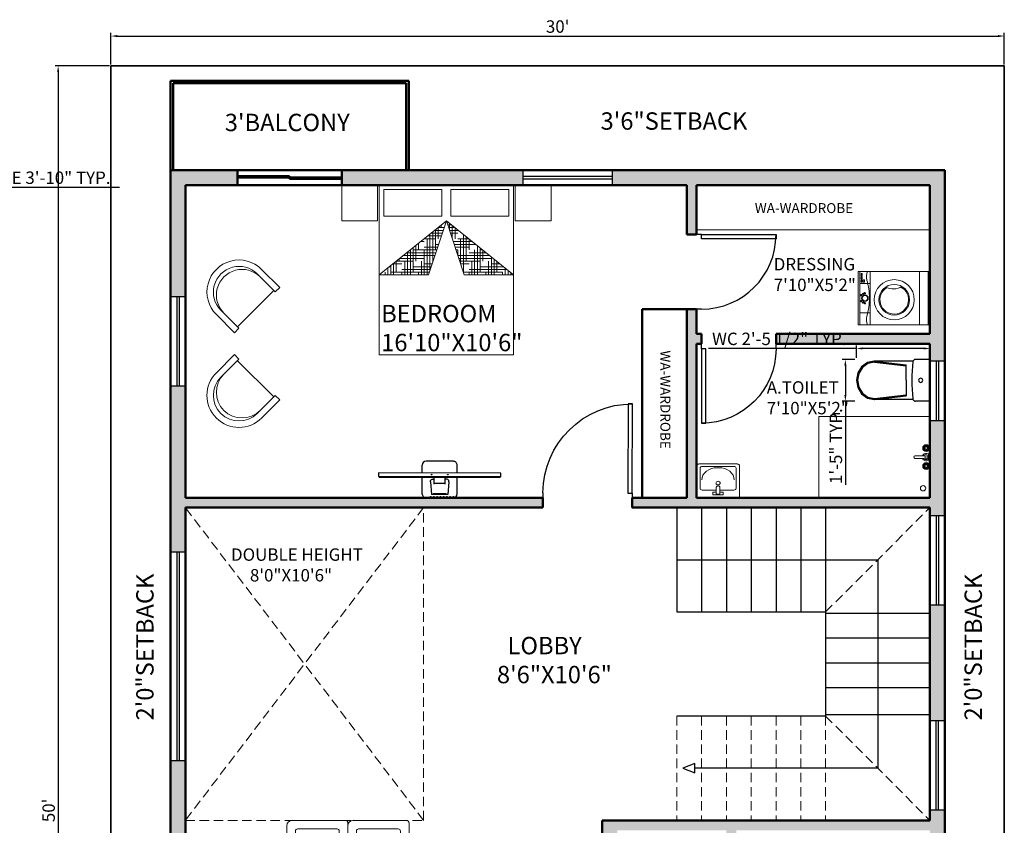
# Model space of a CAD drawing. Units: inches. Extents: x 2638 to 4577, y 1946 to 2619.
# Tile 6 of 8: x 3050 to 3447, y 2294 to 2619. Entities that reach past the tile are written whole.
import ezdxf

# ---------------------------------------------------------------- set-up
doc = ezdxf.new("R2010")
doc.units = ezdxf.units.IN
doc.linetypes.add('DASHED', pattern=[19.05, 12.7, -6.35])
for name, color, linetype, lineweight in [('A-ANNO-DIMS', 2, 'Continuous', 18), ('A-ANNO-TEXT', 7, 'Continuous', 25), ('A-AREA-IDEN', 7, 'Continuous', 25), ('A-DOOR', 4, 'Continuous', 25), ('A-FLOR-FIXT', 8, 'Continuous', 18), ('A-FLOR-OVHD', 8, 'DASHED', 18), ('A-FLOR-STRS', 3, 'Continuous', 25), ('A-FURN', 8, 'Continuous', 18), ('A-GLAZ', 4, 'Continuous', 25), ('A-WALL', 7, 'Continuous', 50), ('A-WALL-PATT', 8, 'Continuous', 13), ('C-PROP', 1, 'Continuous', 35)]:
    doc.layers.add(name, color=color, linetype=linetype, lineweight=lineweight)
doc.layers.add('SANTEH', color=7, linetype='Continuous')
doc.layers.add('window', color=130, linetype='Continuous')
doc.styles.get("Standard").update_dxf_attribs({"font": 'arial.ttf'})
doc.dimstyles.new('ISO-25', dxfattribs={"dimtxt": 5, "dimasz": 2.5, "dimexe": 1.25, "dimexo": 0.625, "dimtad": 1, "dimdec": 1, "dimlunit": 3, "dimtxsty": 'Standard', "dimcen": 2.5, "dimclrt": 1, "dimadec": 0, "dimazin": 0, "dimtfac": 1, "dimtdec": 1, "dimtmove": 0, "dimatfit": 3, "dimfxl": 1, "dimarcsym": 0})

# ---------------------------------------------------------------- blocks, each defined once
blk = doc.blocks.new('*D6')
at = {"layer": 'A-ANNO-DIMS', "color": 0, "lineweight": -2, "transparency": 16777216}
for p, q in [((3086.99, 2600.78), (3086.99, 2613.44)), ((3089.49, 2612.19), (3444.49, 2612.19)), ((3446.99, 2600.78), (3446.99, 2613.44))]:
    blk.add_line(p, q, dxfattribs=at)
at = {"layer": 'A-ANNO-DIMS', "color": 0, "transparency": 16777216}
for points in [[(3089.49, 2612.61), (3089.49, 2611.77), (3086.99, 2612.19)], [(3444.49, 2612.61), (3444.49, 2611.77), (3446.99, 2612.19)]]:
    blk.add_solid(points, dxfattribs=at)
at = {"layer": 'Defpoints', "color": 0, "transparency": 16777216}
for p in [(3446.99, 2612.19), (3086.99, 2600.16), (3446.99, 2600.16)]:
    blk.add_point(p, dxfattribs=at)
at = {"layer": 'A-ANNO-DIMS', "color": 0, "transparency": 16777216, "insert": (3266.99, 2615.37), "char_height": 5, "attachment_point": 5}
blk.add_mtext("30'", dxfattribs=at)
blk = doc.blocks.new('*D7')
at = {"layer": 'A-ANNO-DIMS', "color": 0, "lineweight": -2, "transparency": 16777216}
for p, q in [((3086.37, 2600.16), (3064.44, 2600.16)), ((3065.69, 2597.66), (3065.69, 2002.66)), ((3086.37, 2000.16), (3064.44, 2000.16))]:
    blk.add_line(p, q, dxfattribs=at)
at = {"layer": 'A-ANNO-DIMS', "color": 0, "transparency": 16777216}
for points in [[(3065.28, 2597.66), (3066.11, 2597.66), (3065.69, 2600.16)], [(3065.28, 2002.66), (3066.11, 2002.66), (3065.69, 2000.16)]]:
    blk.add_solid(points, dxfattribs=at)
at = {"layer": 'Defpoints', "color": 0, "transparency": 16777216}
for p in [(3086.99, 2600.16), (3065.69, 2000.16), (3086.99, 2000.16)]:
    blk.add_point(p, dxfattribs=at)
at = {"layer": 'A-ANNO-DIMS', "color": 0, "transparency": 16777216, "insert": (3062.52, 2300.16), "char_height": 5, "attachment_point": 5, "rotation": 90}
blk.add_mtext("50'", dxfattribs=at)
blk = doc.blocks.new('*U5')
for p, q in [((0, 0), (0, -6)), ((30, 0), (30, -6))]:
    blk.add_line(p, q)
blk.add_lwpolyline([(0, 0), (0, 30), (1.75, 30), (1.75, 0)], close=True)
blk.add_arc((0, 0), 30, 0, 90)
blk = doc.blocks.new('*U4')
for p, q in [((0, 0), (0, -6)), ((36, 0), (36, -6))]:
    blk.add_line(p, q)
blk.add_lwpolyline([(0, 0), (0, 36), (1.75, 36), (1.75, 0)], close=True)
blk.add_arc((0, 0), 36, 0, 90)
blk = doc.blocks.new('Rac7')
at = {"color": 0}
for p, q in [((-39501, -24232), (-39501, -23830)), ((-39474, -23808), (-38988, -23808)), ((-39457, -23859), (-39457, -24115)), ((-39032, -23838), (-39430, -23838)), ((-39221, -23855), (-39241, -23855)), ((-39005, -24115), (-39005, -23859)), ((-39005, -23859), (-39005, -23859)), ((-38961, -23830), (-38961, -24232)), ((-39253, -24186), (-39253, -24094)), ((-39209, -24186), (-39209, -24094)), ((-38961, -24232), (-39501, -24232)), ((-39430, -24136), (-39253, -24136)), ((-39297, -24164), (-39253, -24164)), ((-39297, -24194), (-39297, -24164)), ((-39165, -24194), (-39297, -24194)), ((-39253, -24186), (-39209, -24186)), ((-39209, -24136), (-39032, -24136)), ((-39209, -24164), (-39165, -24164)), ((-39165, -24164), (-39165, -24194))]:
    blk.add_line(p, q, dxfattribs=at)
at = {"color": 0, "extrusion": (0, 0, -1)}
for centre, major_axis, start_param, end_param in [((-39474, -23830), (-27, 0), 0, 1.570796), ((-39430, -23859), (-27, 0), 0, 1.570796), ((-39241, -24007), (-194, 0), 0, 1.570796), ((-39221, -24007), (-194, 0), 1.570796, 3.141593), ((-39032, -23859), (-27, 0), 1.570796, 3.141593), ((-38988, -23830), (-27, 0), 1.570796, 3.141593), ((-39430, -24115), (-27, 0), -1.570796, 0), ((-39231, -24104), (-25.3, 0), 0.552816, 2.588777), ((-39032, -24115), (-27, 0), -3.141593, -1.570796)]:
    blk.add_ellipse(centre, major_axis=major_axis, ratio=0.785714, start_param=start_param, end_param=end_param, dxfattribs=at)
blk.add_ellipse((-39231, -24048), major_axis=(-27.9, 0), ratio=0.785714, dxfattribs=at)
blk = doc.blocks.new('WC 2 Symb_109')
at = {"layer": 'SANTEH'}
for p, q in [((0, 0), (0, 380)), ((0, 380), (132.4, 380)), ((153.6, 364.9), (506.8, 364.9)), ((506.3, 364.9), (215.7, 330.9)), ((506.3, 356), (215.7, 322)), ((215.7, 190), (215.7, 330.9)), ((215.7, 190), (215.7, 49.1)), ((153.8, 15.1), (506.8, 15.1)), ((506.3, 24), (215.7, 58)), ((506.3, 15.1), (215.7, 49.1)), ((0, 0), (132.4, 0))]:
    blk.add_line(p, q, dxfattribs=at)
for points in [[(154.6, 360.1), (153.9, 364.1), (152.3, 367.9), (150.2, 371.3), (147.4, 374.3), (144.1, 376.7), (140.5, 378.5), (136.5, 379.6), (132.4, 380)], [(154.6, 19.7), (158.6, 62.1), (161.4, 104.7), (163.1, 147.3), (163.7, 189.9), (163.1, 232.5), (161.4, 275.1), (158.6, 317.7), (154.6, 360.1)], [(506.8, 15.1), (569.2, 28.4), (622.2, 66.3), (657.6, 123.1), (670, 190), (657.6, 256.9), (622.2, 313.7), (569.2, 351.6), (506.8, 364.9)], [(506.3, 24), (565.5, 36.6), (615.7, 72.6), (649.2, 126.5), (661, 190), (649.2, 253.5), (615.7, 307.4), (565.5, 343.4), (506.3, 356)], [(132.4, 0), (136.5, 0.4), (140.4, 1.5), (144.1, 3.2), (147.3, 5.6), (150.1, 8.6), (152.3, 12), (153.8, 15.7), (154.6, 19.7)]]:
    blk.add_lwpolyline(points, dxfattribs=at)
blk.add_lwpolyline([(83.6, 208.5), (70.4, 203.1), (64.9, 190), (70.4, 176.9), (83.6, 171.5), (96.8, 176.9), (102.2, 190), (96.8, 203.1)], close=True, dxfattribs=at)
blk = doc.blocks.new('Faucet - Bathroom top')
for p, q in [((-4.107, 0.125), (-4.375, 0.125)), ((-3.75, 0.4788), (-3.75, 0.75)), ((-3.5, 0.482), (-3.5, 0.75)), ((-3.1461, 0.125), (-2.875, 0.125)), ((3.143, 0.125), (2.875, 0.125)), ((3.5, 0.4788), (3.5, 0.75)), ((3.75, 0.482), (3.75, 0.75)), ((4.1039, 0.125), (4.375, 0.125)), ((-4.1039, -0.125), (-4.375, -0.125)), ((-3.75, -0.4821), (-3.75, -0.75)), ((-3.5, -0.4789), (-3.5, -0.75)), ((-3.143, -0.125), (-2.875, -0.125)), ((-0.5, -0.8639), (-0.5, -4.5)), ((0.5, -4.5), (0.5, -0.8631)), ((3.1461, -0.125), (2.875, -0.125)), ((3.5, -0.4821), (3.5, -0.75)), ((3.75, -0.4789), (3.75, -0.75)), ((4.107, -0.125), (4.375, -0.125))]:
    blk.add_line(p, q)
for centre, radius in [((-3.625, 0), 1.375), ((-4.625, 0), 0.2795), ((-3.625, 0), 0.5), ((-3.625, 1), 0.2795), ((-2.625, 0), 0.2795), ((0, 0), 0.5), ((3.625, 0), 1.375), ((2.625, 0), 0.2795), ((3.625, 0), 0.5), ((3.625, 1), 0.2795), ((4.625, 0), 0.2795), ((-3.625, -1), 0.2795), ((3.625, -1), 0.2795)]:
    blk.add_circle(centre, radius)
for centre, radius, start, end in [((-3.625, 0), 1, 105.2407, 164.2093), ((-3.625, 0), 1, 16.44125, 74.07887), ((0, 0), 1.5, 289.6514, 250.3603), ((0, 0), 1, 300.3431, 239.7554), ((3.625, 0), 1, 106.12, 164.0884), ((3.625, 0), 1, 16.23422, 73.90469), ((-3.625, 0), 1, 196.2342, 253.9047), ((-3.625, 0), 1, 286.12, 344.0884), ((3.625, 0), 1, 196.4413, 254.0789), ((3.625, 0), 1, 285.2407, 344.2093), ((0, -4.5), 0.5, 180, 0)]:
    blk.add_arc(centre, radius, start, end)
blk = doc.blocks.new('*X22')
at = {"color": 0}
for p, q in [((20.188, 14.75), (20.188, 14.767)), ((20.199, 14.781), (20.277, 14.781)), ((20.25, 14.812), (20.277, 14.812)), ((20.094, 14.375), (20.094, 14.65)), ((20.098, 14.656), (20.125, 14.656)), ((20.124, 14.688), (20.25, 14.688)), ((20.125, 14.5), (20.125, 14.689)), ((20.149, 14.719), (20.277, 14.719)), ((20.156, 14.625), (20.156, 14.728)), ((20.174, 14.75), (20.277, 14.75)), ((20.25, 14.319), (20.25, 14.75)), ((20.023, 14.562), (20.277, 14.562)), ((20.031, 14.247), (20.031, 14.573)), ((20.062, 14.257), (20.062, 14.612)), ((20.125, 14.594), (20.277, 14.594)), ((20.219, 14.309), (20.219, 14.625)), ((20.25, 14.625), (20.277, 14.625)), ((19.922, 14.438), (20, 14.438)), ((19.948, 14.469), (20.125, 14.469)), ((19.973, 14.5), (20.25, 14.5)), ((19.998, 14.531), (20.277, 14.531)), ((20, 14.237), (20, 14.5)), ((20.188, 14.299), (20.188, 14.5)), ((20.25, 14.438), (20.277, 14.438)), ((19.844, 14.185), (19.844, 14.34)), ((19.875, 14.25), (19.875, 14.379)), ((19.875, 14.344), (20.277, 14.344)), ((19.906, 14.375), (19.906, 14.417)), ((19.969, 14.226), (19.969, 14.375)), ((20, 14.375), (20.277, 14.375)), ((20.125, 14.406), (20.277, 14.406)), ((20.156, 14.288), (20.156, 14.375)), ((19.746, 14.219), (19.875, 14.219)), ((19.75, 14.154), (19.75, 14.223)), ((19.772, 14.25), (20, 14.25)), ((19.781, 14.164), (19.781, 14.262)), ((19.797, 14.281), (20.125, 14.281)), ((19.812, 14.174), (19.812, 14.301)), ((19.822, 14.312), (20.229, 14.312)), ((19.938, 14.216), (19.938, 14.25)), ((19.719, 14.073), (19.719, 14.114)), ((19.721, 14.188), (19.75, 14.188)), ((19.75, 14.034), (19.75, 14.103)), ((19.702, 14.094), (19.779, 14.094)), ((19.727, 14.062), (19.873, 14.062)), ((19.752, 14.031), (19.875, 14.031)), ((19.781, 13.995), (19.781, 14.093)), ((19.812, 14), (19.812, 14.082)), ((19.875, 13.878), (19.875, 14)), ((19.906, 13.84), (19.906, 14.051)), ((19.938, 13.801), (19.938, 14.041)), ((19.969, 13.875), (19.969, 14.031)), ((20, 14), (20, 14.02)), ((20, 14), (20.061, 14)), ((20.062, 13.645), (20.062, 14)), ((20.094, 13.625), (20.094, 13.989)), ((19.827, 13.938), (20.25, 13.938)), ((19.853, 13.906), (20.125, 13.906)), ((19.875, 13.969), (20.156, 13.969)), ((19.878, 13.875), (20, 13.875)), ((20.031, 13.684), (20.031, 13.875)), ((20.125, 13.75), (20.125, 13.979)), ((20.156, 13.875), (20.156, 13.969)), ((20.219, 13.451), (20.219, 13.875)), ((20.25, 13.5), (20.25, 13.937)), ((20.25, 13.875), (20.277, 13.875)), ((19.953, 13.781), (20.277, 13.781)), ((20, 13.812), (20.277, 13.812)), ((20.125, 13.844), (20.277, 13.844)), ((19.978, 13.75), (20.25, 13.75)), ((20, 13.723), (20, 13.75)), ((20.003, 13.719), (20.125, 13.719)), ((20.125, 13.656), (20.277, 13.656)), ((20.188, 13.49), (20.188, 13.75)), ((20.25, 13.688), (20.277, 13.688)), ((20.079, 13.625), (20.277, 13.625)), ((20.104, 13.594), (20.277, 13.594)), ((20.129, 13.562), (20.25, 13.562)), ((20.156, 13.529), (20.156, 13.625)), ((20.205, 13.469), (20.277, 13.469)), ((20.23, 13.438), (20.277, 13.438)), ((20.25, 13.5), (20.277, 13.5)), ((20.255, 13.406), (20.277, 13.406))]:
    blk.add_line(p, q, dxfattribs=at)
blk = doc.blocks.new('MAT-P02')
for p, q in [((-1.17, 0), (-1.17, -0.4)), ((-1.17, 0), (-0.77, 0)), ((-0.77, 0), (-0.77, -0.4)), ((-0.75, 0), (0.75, 0)), ((-0.75, 0), (-0.75, -1.9)), ((0.75, 0), (0.75, -1.9)), ((0.77, 0), (1.17, 0)), ((0.77, 0), (0.77, -0.4)), ((1.17, 0), (1.17, -0.4)), ((-0.7, -0.05), (-0.7, -0.35)), ((-0.7, -0.05), (-0.05, -0.05)), ((-0.05, -0.35), (-0.05, -0.05)), ((0.05, -0.05), (0.7, -0.05)), ((0.05, -0.35), (0.05, -0.05)), ((0.7, -0.05), (0.7, -0.35)), ((-1.17, -0.4), (-0.77, -0.4)), ((-0.75, -1.003), (0, -0.4)), ((0, -0.4), (-0.75, -1.003)), ((-0.7, -0.35), (-0.05, -0.35)), ((0, -0.4), (-0.2, -1.003)), ((0, -0.4), (0.2, -1.003)), ((0, -0.4), (0.75, -1.003)), ((0.05, -0.35), (0.7, -0.35)), ((0.77, -0.4), (1.17, -0.4)), ((-0.75, -1.003), (-0.2, -1.003)), ((0.2, -1.003), (0.75, -1.003)), ((0.75, -1.9), (-0.75, -1.9))]:
    blk.add_line(p, q)
at = {"xscale": -1, "rotation": 90}
blk.add_blockref('*X22', (14.128, 19.274), dxfattribs=at)
blk = doc.blocks.new('12PSTG07')
at = {"color": 0, "linetype": 'ByBlock'}
for p, q in [((0, 15), (-12, 15)), ((0, 12), (0, 15)), ((-12, 12), (0, 12)), ((-1, -12), (-1, 12)), ((-12, -12), (0, -12)), ((0, -12), (0, -15)), ((0, -15), (-12, -15))]:
    blk.add_line(p, q, dxfattribs=at)
for centre, radius in [((-12, 0), 15), ((-12, 0), 12), ((-10, 0), 12)]:
    blk.add_arc(centre, radius, 90, 270, dxfattribs=at)
blk = doc.blocks.new('sofa-27')
at = {"color": 0, "linetype": 'ByBlock'}
for p, q in [((-0.059, 0.059), (-0.059, 0.49)), ((0.035, 0.118), (0.035, 0.461)), ((0.094, 0.52), (0.459, 0.52)), ((0.518, 0.118), (0.518, 0.461)), ((0.613, 0.03), (0.613, 0.49)), ((0.583, 0), (0, 0)), ((0.494, 0.094), (0.059, 0.094))]:
    blk.add_line(p, q, dxfattribs=at)
for centre, radius, start, end in [((-0.03, 0.49), 0.0295, 90, 180), ((-0.024, 0.461), 0.0591, 360, 90), ((0.094, 0.461), 0.0591, 90, 180), ((0.459, 0.461), 0.0591, 0, 90), ((0.577, 0.461), 0.0591, 90, 180), ((0.583, 0.49), 0.0295, 0, 90), ((0.059, 0.118), 0.0236, 180, 270), ((0.494, 0.118), 0.0236, 270, 0), ((0, 0.059), 0.0591, 180, 270), ((0.583, 0.03), 0.0295, 270, 0)]:
    blk.add_arc(centre, radius, start, end, dxfattribs=at)
blk = doc.blocks.new('TV')
at = {"color": 0}
for p, q in [((3967.27, 1784.85), (3967.05, 1784.65)), ((3967.76, 1763.68), (3967.54, 1763.86))]:
    blk.add_line(p, q, dxfattribs=at)
at = {"layer": 'window'}
for p, q in [((3967.54, 1763.86), (3967.05, 1784.65)), ((3964.41, 1777.23), (3967.22, 1777.3)), ((3968.01, 1777.32), (3969.36, 1777.35)), ((3966.53, 1775.82), (3964.33, 1775.61)), ((3964.34, 1775.34), (3964.45, 1775.34)), ((3964.34, 1775.31), (3964.43, 1775.32)), ((3966.14, 1775.2), (3967.01, 1775.22)), ((3966.14, 1775.18), (3967.27, 1775.2)), ((3966.14, 1775.18), (3966.14, 1775.2)), ((3966.3, 1773.29), (3966.26, 1775.18)), ((3966.19, 1773.28), (3967.31, 1773.31)), ((3966.19, 1773.26), (3967.05, 1773.28)), ((3966.19, 1773.26), (3966.19, 1773.28)), ((3964.39, 1773.06), (3964.48, 1773.06)), ((3964.39, 1773.04), (3964.5, 1773.04)), ((3966.61, 1772.66), (3964.4, 1772.77)), ((3964.55, 1771.15), (3967.36, 1771.22)), ((3968.15, 1771.24), (3969.5, 1771.27))]:
    blk.add_line(p, q, dxfattribs=at)
for points in [[(3968.33, 1763.69), (3967.83, 1784.86), (3967.27, 1784.85), (3967.76, 1763.68), (3968.33, 1763.69)], [(3963.86, 1771.81), (3963.75, 1776.54)], [(3970.16, 1771.96), (3970.05, 1776.69)], [(3964.4, 1772.77), (3964.33, 1775.61)], [(3964.48, 1773.06), (3964.43, 1775.32)], [(3964.5, 1773.04), (3964.45, 1775.34)]]:
    blk.add_lwpolyline(points, dxfattribs=at)
for points in [[(3966.53, 1775.82, -0.263666), (3966.93, 1775.69), (3967, 1775.57), (3967.01, 1775.22)], [(3966.61, 1772.66, 0.263666), (3967, 1772.81), (3967.06, 1772.93), (3967.05, 1773.28)]]:
    blk.add_lwpolyline(points, format="xyb", dxfattribs=at)
for centre, radius in [((3963.91, 1775.73), 0.0679), ((3963.93, 1775.17), 0.0679), ((3967.77, 1775.68), 0.0451), ((3963.94, 1774.6), 0.0679), ((3963.95, 1774.04), 0.0679), ((3963.97, 1773.48), 0.0679), ((3963.98, 1772.92), 0.0679), ((3963.99, 1772.35), 0.0679), ((3964.01, 1771.79), 0.0679), ((3967.83, 1772.86), 0.0451)]:
    blk.add_circle(centre, radius, dxfattribs=at)
for centre, start, end in [((3964.42, 1776.56), 91.3414, 181.3414), ((3969.38, 1776.67), 1.3414, 91.3414), ((3964.53, 1771.83), 181.3414, 271.3414), ((3969.49, 1771.94), 271.3414, 1.3414)]:
    blk.add_arc(centre, 0.676, start, end, dxfattribs=at)
blk = doc.blocks.new('WIN-36')
for p, q in [((2761.41, 2540.16), (2761.41, 2534.16)), ((2797.41, 2540.16), (2797.41, 2534.16)), ((2761.41, 2537.66), (2797.41, 2537.66)), ((2761.41, 2536.66), (2797.41, 2536.66))]:
    blk.add_line(p, q)
blk = doc.blocks.new('WIN-24')
for p, q in [((2905.41, 2558.16), (2905.41, 2552.16)), ((2905.41, 2555.66), (2929.41, 2555.66)), ((2929.41, 2558.16), (2929.41, 2552.16)), ((2905.41, 2554.66), (2929.41, 2554.66))]:
    blk.add_line(p, q)
blk = doc.blocks.new('WIN-84')
for p, q in [((2695.41, 2404.16), (2689.41, 2404.16)), ((2691.91, 2404.16), (2691.91, 2320.16)), ((2692.91, 2404.16), (2692.91, 2320.16)), ((2695.41, 2320.16), (2689.41, 2320.16))]:
    blk.add_line(p, q)
blk = doc.blocks.new('*D69')
at = {"layer": 'A-ANNO-DIMS', "color": 0, "lineweight": -2, "transparency": 16777216}
for p, q in [((3387.38, 2486.31), (3327.72, 2486.31)), ((3387.38, 2482.49), (3387.38, 2487.56)), ((3414.49, 2486.31), (3389.88, 2486.31)), ((3416.99, 2482.49), (3416.99, 2487.56))]:
    blk.add_line(p, q, dxfattribs=at)
at = {"layer": 'A-ANNO-DIMS', "color": 0, "transparency": 16777216}
for points in [[(3389.88, 2486.72), (3389.88, 2485.89), (3387.38, 2486.31)], [(3414.49, 2486.72), (3414.49, 2485.89), (3416.99, 2486.31)]]:
    blk.add_solid(points, dxfattribs=at)
at = {"layer": 'Defpoints', "color": 0, "transparency": 16777216}
for p in [(3387.38, 2486.31), (3387.38, 2481.86), (3416.99, 2481.86)]:
    blk.add_point(p, dxfattribs=at)
at = {"layer": 'A-ANNO-DIMS', "color": 1, "transparency": 16777216, "insert": (3356.3, 2489.52), "char_height": 5, "attachment_point": 5}
blk.add_mtext('WC 2\'-5 1/2" TYP.', dxfattribs=at)
blk = doc.blocks.new('*D70')
at = {"layer": 'A-ANNO-DIMS', "color": 0, "lineweight": -2, "transparency": 16777216}
for p, q in [((3386.76, 2481.86), (3381.69, 2481.86)), ((3382.94, 2479.36), (3382.94, 2467.57)), ((3386.76, 2465.07), (3381.69, 2465.07)), ((3382.94, 2465.07), (3382.94, 2431.32))]:
    blk.add_line(p, q, dxfattribs=at)
at = {"layer": 'A-ANNO-DIMS', "color": 0, "transparency": 16777216}
for points in [[(3382.53, 2479.36), (3383.36, 2479.36), (3382.94, 2481.86)], [(3382.53, 2467.57), (3383.36, 2467.57), (3382.94, 2465.07)]]:
    blk.add_solid(points, dxfattribs=at)
at = {"layer": 'Defpoints', "color": 0, "transparency": 16777216}
for p in [(3387.38, 2481.86), (3382.94, 2465.07), (3387.38, 2465.07)]:
    blk.add_point(p, dxfattribs=at)
at = {"layer": 'A-ANNO-DIMS', "color": 1, "transparency": 16777216, "insert": (3379.76, 2446.94), "char_height": 5, "attachment_point": 5, "rotation": 90}
blk.add_mtext('1\'-5" TYP.', dxfattribs=at)
blk = doc.blocks.new('*D79')
at = {"layer": 'A-ANNO-DIMS', "color": 0, "lineweight": -2, "transparency": 16777216}
for p, q in [((2936.51, 2557.53), (2936.51, 2549.99)), ((2982.61, 2557.53), (2982.61, 2549.99)), ((2939.01, 2551.24), (2980.11, 2551.24)), ((2982.61, 2551.24), (3090.4, 2551.24))]:
    blk.add_line(p, q, dxfattribs=at)
at = {"layer": 'A-ANNO-DIMS', "color": 0, "transparency": 16777216}
for points in [[(2939.01, 2551.66), (2939.01, 2550.82), (2936.51, 2551.24)], [(2980.11, 2551.66), (2980.11, 2550.82), (2982.61, 2551.24)]]:
    blk.add_solid(points, dxfattribs=at)
at = {"layer": 'Defpoints', "color": 0, "transparency": 16777216}
for p in [(2936.51, 2558.16), (2982.61, 2558.16), (2982.61, 2551.24)]:
    blk.add_point(p, dxfattribs=at)
at = {"layer": 'A-ANNO-DIMS', "color": 1, "transparency": 16777216, "insert": (3037.75, 2554.45), "char_height": 5, "attachment_point": 5}
blk.add_mtext('WASHING MACHINE 3\'-10" TYP.', dxfattribs=at)

msp = doc.modelspace()

# ---------------------------------------------------------------- hatches: boundary and pattern name
at = {"layer": 'A-WALL-PATT', "transparency": 33554687}
h = msp.add_hatch(color=256, dxfattribs=at)
h.dxf.hatch_style = 1
h.paths.add_polyline_path([(3116.99, 2552.16), (3137.99, 2552.16), (3137.99, 2558.16), (3110.99, 2558.16), (3110.99, 2507.16), (3116.99, 2507.16)])
h.paths.add_polyline_path([(3252.94, 2558.16), (3179.99, 2558.16), (3179.99, 2552.16), (3194.4, 2552.16), (3252.94, 2552.16)])
h.paths.add_polyline_path([(3422.99, 2558.16), (3288.94, 2558.16), (3288.94, 2552.16), (3318.99, 2552.16), (3318.99, 2532.16), (3322.99, 2532.16), (3322.99, 2552.16), (3416.99, 2552.16), (3416.99, 2492.16), (3354.99, 2492.16), (3354.99, 2488.16), (3416.99, 2488.16), (3416.99, 2481.16), (3422.99, 2481.16)])
h.paths.add_polyline_path([(3422.99, 2457.16), (3416.99, 2457.16), (3416.99, 2426.16), (3372.26, 2426.16), (3322.99, 2426.16), (3322.99, 2439.06), (3322.99, 2488.16), (3324.99, 2488.16), (3324.99, 2492.16), (3322.99, 2492.16), (3322.99, 2502.16), (3318.99, 2502.16), (3318.99, 2426.16), (3297.01, 2426.16), (3296.99, 2422.16), (3416.99, 2422.16), (3416.99, 2418.91), (3422.99, 2418.91)])
h.paths.add_polyline_path([(3146.99, 2104.16), (3116.99, 2104.16), (3116.99, 2116.16), (3110.99, 2116.16), (3110.99, 2098.16), (3146.99, 2098.16)])
h.paths.add_polyline_path([(3236.99, 2104.16), (3224.99, 2104.16), (3224.99, 2098.16), (3236.99, 2098.16)])
h.paths.add_polyline_path([(3290.99, 2252.16), (3284.99, 2252.16), (3284.99, 2104.16), (3278.99, 2104.16), (3278.99, 2098.16), (3284.99, 2098.16), (3284.99, 2000.16), (3290.99, 2000.16), (3290.99, 2018.16), (3314.99, 2018.16), (3314.99, 2024.16), (3290.99, 2024.16)])
h.paths.add_polyline_path([(3422.99, 2060.16), (3416.99, 2060.16), (3416.99, 2024.16), (3392.99, 2024.16), (3392.99, 2018.16), (3422.99, 2018.16)])
h.paths.add_polyline_path([(3422.99, 2244.16), (3416.99, 2244.16), (3416.99, 2220.16), (3372.26, 2220.16), (3338.99, 2220.16), (3338.99, 2222.16), (3334.99, 2222.16), (3334.99, 2216.16), (3416.99, 2216.16), (3416.99, 2096.16), (3422.99, 2096.16)])
h.paths.add_polyline_path([(3422.99, 2300.41), (3416.99, 2300.41), (3416.99, 2296.16), (3284.99, 2296.16), (3284.99, 2288.16), (3290.99, 2288.16), (3290.99, 2292.16), (3334.99, 2292.16), (3334.99, 2252.16), (3338.99, 2252.16), (3338.99, 2292.16), (3416.99, 2292.16), (3416.99, 2268.16), (3422.99, 2268.16)])
h.paths.add_polyline_path([(3422.99, 2382.91), (3416.99, 2382.91), (3416.99, 2336.41), (3422.99, 2336.41)])
h.paths.add_polyline_path([(3260.99, 2426.16), (3116.99, 2426.16), (3116.99, 2471.16), (3110.99, 2471.16), (3110.99, 2404.16), (3116.99, 2404.16), (3116.99, 2422.16), (3260.99, 2422.16)])
h.paths.add_polyline_path([(3116.99, 2320.16), (3110.99, 2320.16), (3110.99, 2152.16), (3116.99, 2152.16)])
h.paths.add_polyline_path([(3192.92, 2481.2), (3252.23, 2481.2), (3252.23, 2507.82), (3192.92, 2507.82)], flags=9)
h.paths.add_polyline_path([(3352.38, 2202.6), (3398.15, 2202.6), (3398.15, 2210.84), (3352.38, 2210.84)], flags=25)
h.paths.add_polyline_path([(3108.13, 2334.43), (3108.13, 2401.53), (3093.19, 2401.53), (3093.19, 2334.43)], flags=9)
h.paths.add_polyline_path([(3441.94, 2334.43), (3441.94, 2401.53), (3426.99, 2401.53), (3426.99, 2334.43)], flags=9)
h.paths.add_polyline_path([(3282.12, 2570.46), (3349.22, 2570.46), (3349.22, 2585.4), (3282.12, 2585.4)], flags=9)
h.paths.add_polyline_path([(3240.15, 2347.41), (3289.11, 2347.41), (3289.11, 2374.03), (3240.15, 2374.03)], flags=9)
h.paths.add_polyline_path([(3169.91, 2226.85), (3224.05, 2226.85), (3224.05, 2253.46), (3169.91, 2253.46)], flags=9)
h.paths.add_polyline_path([(3209.4, 2038.68), (3263.9, 2038.68), (3263.9, 2065.29), (3209.4, 2065.29)], flags=9)
h.paths.add_polyline_path([(3313.05, 2123.44), (3369.27, 2123.44), (3369.27, 2150.05), (3313.05, 2150.05)], flags=9)
h.paths.add_polyline_path([(3359.46, 2259.32), (3395.23, 2259.32), (3395.23, 2278.33), (3359.46, 2278.33)], flags=25)

# ---------------------------------------------------------------- linework, layer by layer
at = {"layer": 'A-FLOR-FIXT'}
for p, q in [((3416.99, 2517.31), (3388.1, 2517.31)), ((3388.1, 2495.85), (3388.1, 2517.31)), ((3388.79, 2495.85), (3388.79, 2517.31)), ((3392.94, 2495.85), (3392.94, 2517.31)), ((3412.84, 2495.85), (3412.84, 2517.31)), ((3416.3, 2495.85), (3416.3, 2517.31)), ((3416.99, 2495.85), (3416.99, 2517.31)), ((3392.94, 2512.46), (3388.79, 2512.46)), ((3392.94, 2500.7), (3388.79, 2500.7)), ((3416.99, 2495.85), (3388.1, 2495.85))]:
    msp.add_line(p, q, dxfattribs=at)
for points in [[(3389.25, 2515.65), (3389.25, 2516.55), (3389.76, 2516.55), (3389.76, 2515.65)], [(3389.25, 2514.34), (3389.25, 2515.24), (3389.76, 2515.24), (3389.76, 2514.34)], [(3389.25, 2513.02), (3389.25, 2513.92), (3389.76, 2513.92), (3389.76, 2513.02)], [(3390.13, 2513.02), (3390.13, 2513.92), (3390.63, 2513.92), (3390.63, 2513.02)]]:
    msp.add_lwpolyline(points, close=True, dxfattribs=at)
at = {"layer": 'A-FLOR-FIXT', "ltscale": 5}
msp.add_lwpolyline([(3372.26, 2426.16), (3416.99, 2426.16), (3416.99, 2458.89), (3372.26, 2458.89)], close=True, dxfattribs=at)
at = {"layer": 'A-FLOR-FIXT'}
for centre, radius in [((3402.63, 2505.93), 8.1), ((3402.63, 2505.93), 6.17), ((3389.32, 2507.83), 0.271), ((3390.84, 2506.58), 1.34), ((3390.05, 2508.31), 0.271), ((3390.84, 2508.57), 0.271), ((3389.32, 2505.31), 0.271), ((3390.84, 2506.58), 1.07), ((3390.05, 2504.78), 0.271), ((3390.84, 2504.53), 0.271)]:
    msp.add_circle(centre, radius, dxfattribs=at)
at = {"layer": 'A-FLOR-FIXT', "ltscale": 5}
msp.add_circle((3414.24, 2429.96), 1.06, dxfattribs=at)
at = {"layer": 'A-FLOR-FIXT'}
for centre, radius, start, end in [((3396.3, 2515.23), 4.89, 154.895, 196.6068), ((3362.73, 2506.05), 29.92, 1.0206, 15.0937), ((3402.63, 2505.93), 5.77, 121.8067, 62.1506), ((3402.24, 2517.13), 6.83, 243.19, 300.7673), ((3362.73, 2507.11), 29.92, 344.9063, 358.9794), ((3396.3, 2497.92), 4.89, 163.3932, 205.105)]:
    msp.add_arc(centre, radius, start, end, dxfattribs=at)
at = {"layer": 'A-FLOR-OVHD', "ltscale": 0.3}
for p, q in [((3212.99, 2296.16), (3116.99, 2422.16)), ((3212.99, 2422.16), (3116.99, 2296.16)), ((3212.99, 2296.16), (3212.99, 2422.16)), ((3374.99, 2380.16), (3416.99, 2422.16)), ((3314.99, 2338.16), (3314.99, 2296.16)), ((3324.99, 2338.16), (3324.99, 2296.16)), ((3334.99, 2338.16), (3334.99, 2296.16)), ((3344.99, 2338.16), (3344.99, 2296.16)), ((3354.99, 2338.16), (3354.99, 2296.16)), ((3364.99, 2338.16), (3364.99, 2296.16)), ((3374.99, 2338.16), (3374.99, 2296.16)), ((3374.99, 2338.16), (3416.99, 2296.16)), ((3116.99, 2296.16), (3212.99, 2296.16))]:
    msp.add_line(p, q, dxfattribs=at)
at = {"layer": 'A-FLOR-STRS'}
for p, q in [((3314.99, 2422.16), (3314.99, 2380.16)), ((3324.99, 2422.16), (3324.99, 2380.16)), ((3334.99, 2422.16), (3334.99, 2380.16)), ((3344.99, 2422.16), (3344.99, 2380.16)), ((3354.99, 2422.16), (3354.99, 2380.16)), ((3364.99, 2422.16), (3364.99, 2380.16)), ((3374.99, 2422.16), (3374.99, 2338.16)), ((3314.99, 2380.16), (3374.99, 2380.16)), ((3374.99, 2379.66), (3416.99, 2379.66)), ((3374.99, 2369.66), (3416.99, 2369.66)), ((3374.99, 2359.66), (3416.99, 2359.66)), ((3374.99, 2349.66), (3416.99, 2349.66)), ((3374.99, 2338.16), (3314.99, 2338.16)), ((3416.99, 2338.66), (3374.99, 2338.66))]:
    msp.add_line(p, q, dxfattribs=at)
msp.add_lwpolyline([(3314.99, 2401.16), (3395.99, 2401.16), (3395.99, 2317.16), (3322.22, 2317.16)], dxfattribs=at)
msp.add_lwpolyline([(3317.45, 2317.16), (3322.22, 2315.29), (3322.22, 2319.03)], close=True, dxfattribs=at)
at = {"layer": 'A-FURN'}
msp.add_line((3322.99, 2534.16), (3416.99, 2534.16), dxfattribs=at)
at = {"layer": 'A-WALL'}
for p, q in [((3110.99, 2000.16), (3110.99, 2594.16)), ((3110.99, 2594.16), (3206.99, 2594.16)), ((3111.99, 2593.16), (3205.99, 2593.16)), ((3111.99, 2558.16), (3111.99, 2593.16)), ((3205.99, 2558.16), (3205.99, 2593.16)), ((3206.99, 2558.16), (3206.99, 2594.16)), ((3110.99, 2558.16), (3422.99, 2558.16)), ((3137.99, 2558.16), (3137.99, 2552.16)), ((3137.99, 2555.66), (3158.99, 2555.66)), ((3158.99, 2555.66), (3158.99, 2554.66)), ((3179.99, 2558.16), (3179.99, 2552.16)), ((3422.99, 2558.16), (3422.99, 2018.16)), ((3116.99, 2552.16), (3318.99, 2552.16)), ((3116.99, 2426.16), (3116.99, 2552.16)), ((3137.99, 2555.16), (3179.99, 2555.16)), ((3158.99, 2554.66), (3179.99, 2554.66)), ((3318.99, 2552.16), (3318.99, 2532.16)), ((3322.99, 2552.16), (3322.99, 2532.16)), ((3322.99, 2552.16), (3416.99, 2552.16)), ((3416.99, 2552.16), (3416.99, 2492.16)), ((3318.99, 2532.16), (3322.99, 2532.16)), ((3300.99, 2502.16), (3300.99, 2426.16)), ((3300.99, 2502.16), (3322.99, 2502.16)), ((3318.99, 2502.16), (3318.99, 2426.16)), ((3322.99, 2502.16), (3322.99, 2492.16)), ((3322.99, 2492.16), (3324.99, 2492.16)), ((3324.99, 2492.16), (3324.99, 2488.16)), ((3354.99, 2492.16), (3354.99, 2488.16)), ((3354.99, 2492.16), (3416.99, 2492.16)), ((3322.99, 2488.16), (3322.99, 2426.16)), ((3322.99, 2488.16), (3324.99, 2488.16)), ((3354.99, 2488.16), (3416.99, 2488.16)), ((3416.99, 2488.16), (3416.99, 2426.16)), ((3116.99, 2426.16), (3260.99, 2426.16)), ((3260.99, 2426.16), (3260.99, 2422.16)), ((3296.99, 2426.16), (3296.99, 2422.16)), ((3296.99, 2426.16), (3318.99, 2426.16)), ((3322.99, 2426.16), (3416.99, 2426.16)), ((3116.99, 2422.16), (3260.99, 2422.16)), ((3116.99, 2104.16), (3116.99, 2422.16)), ((3296.99, 2422.16), (3416.99, 2422.16)), ((3416.99, 2422.16), (3416.99, 2296.16)), ((3284.99, 2296.16), (3284.99, 2288.16)), ((3416.99, 2296.16), (3284.99, 2296.16))]:
    msp.add_line(p, q, dxfattribs=at)
at = {"layer": 'C-PROP'}
msp.add_lwpolyline([(3086.99, 2600.16), (3446.99, 2600.16), (3446.99, 2000.16), (3086.99, 2000.16)], close=True, dxfattribs=at)

# ---------------------------------------------------------------- block references
at = {"layer": 'A-DOOR', "rotation": 270}
msp.add_blockref('*U5', (3324.99, 2532.16), dxfattribs=at)
at = {"layer": 'A-DOOR', "xscale": -1}
for name, p, rotation in [('*U5', (3324.99, 2486.16), 180), ('*U4', (3297.02, 2427.95), 359.6786649249896)]:
    msp.add_blockref(name, p, dxfattribs=dict(at, rotation=rotation))
at = {"layer": 'A-FLOR-FIXT', "xscale": 0.0441898926459964, "yscale": 0.0441898926459964, "zscale": 0.0441898926459964, "rotation": 180}
msp.add_blockref('WC 2 Symb_109', (3416.99, 2481.86), dxfattribs=at)
at = {"layer": 'A-FLOR-FIXT', "rotation": 270}
msp.add_blockref('Faucet - Bathroom top', (3415.49, 2442.52), dxfattribs=at)
at = {"layer": 'A-FLOR-FIXT', "xscale": -0.0320670790485951, "yscale": 0.0320670790485951, "zscale": 0.0320670790485951}
msp.add_blockref('Rac7', (2073.61, 3203.21), dxfattribs=at)
at = {"layer": 'A-FURN', "xscale": 36.03633950593442, "yscale": 36.03633950593442, "zscale": 36.03633950593442}
msp.add_blockref('MAT-P02', (3222.15, 2552.16), dxfattribs=at)
at = {"layer": 'A-FURN'}
for name, p, xscale, yscale, zscale, rotation in [('12PSTG07', (3145.87, 2501.76), -0.8597921787217943, 0.8597921787217943, 0.8597921787217943, 135.0000000000001), ('12PSTG07', (3145.87, 2474.69), 0.8597921787217943, 0.8597921787217943, 0.8597921787217943, 44.99999999999996), ('TV', (7112.62, -6900.87), 2.327319231123021, 2.327319231123021, 2.327319231123021, 88.54308451816132), ('sofa-27', (3160.01, 2296.16), -36.66436083614781, 36.66436083614781, 36.66436083614781, 180), ('sofa-27', (3184.63, 2296.16), -36.66436083614781, 36.66436083614781, 36.66436083614781, 180)]:
    msp.add_blockref(name, p, dxfattribs=dict(at, xscale=xscale, yscale=yscale, zscale=zscale, rotation=rotation))
at = {"layer": 'A-GLAZ'}
for name, p in [('WIN-36', (491.53, 18)), ('WIN-84', (421.58, 0))]:
    msp.add_blockref(name, p, dxfattribs=at)
for name, p, rotation in [('WIN-36', (576.83, 5268.57), 270.0000000000014), ('WIN-24', (864.83, 5386.57), 270.0000000000082), ('WIN-36', (882.83, 5180.32), 270.0000000000045), ('WIN-36', (5957.15, -461), 90.00000000000684)]:
    msp.add_blockref(name, p, dxfattribs=dict(at, rotation=rotation))

# ---------------------------------------------------------------- texts
at = {"layer": 'A-ANNO-TEXT', "attachment_point": 1}
for s, width, insert, char_height in [("{\\fTimes New Roman|b0|i0|c0|p18;3'BALCONY}", 61.0557, (3132.85, 2580.87), 7), ('{\\fTimes New Roman|b0|i0|c0|p18;3\'6"SETBACK}', 61.0557, (3284.29, 2581.44), 7), ('WA-WARDROBE', 29.5334, (3346.44, 2544.86), 4)]:
    msp.add_mtext_dynamic_manual_height_columns(s, width=width, gutter_width=12.5, heights=[0], dxfattribs=dict(at, insert=insert, char_height=char_height))
for s, width, insert, char_height, rotation in [('WA-WARDROBE', 29.5334, (3312.4, 2485.51), 4, 270), ('{\\fTimes New Roman|b0|i0|c0|p18;2\'0"SETBACK}', 61.0557, (3097.15, 2336.4), 7, 90), ('{\\fTimes New Roman|b0|i0|c0|p18;2\'0"SETBACK}', 61.0557, (3430.96, 2336.4), 7, 90)]:
    msp.add_mtext_dynamic_manual_height_columns(s, width=width, gutter_width=12.5, heights=[0], dxfattribs=dict(at, insert=insert, char_height=char_height, rotation=rotation))
at = {"layer": 'A-AREA-IDEN', "attachment_point": 1}
for s, width, insert, char_height in [('{\\fTimes New Roman|b0|i0|c0|p18;DRESSING\\P7\'10"X5\'2"}', 61.0557, (3354.06, 2522.76), 5), ('{\\fTimes New Roman|b0|i0|c0|p18;BEDROOM\\P16\'10"X10\'6"}', 61.0557, (3195.88, 2503.86), 7), ('{\\fTimes New Roman|b0|i0|c0|p18;A.TOILET\\P7\'10"X5\'2"}', 61.0557, (3351.26, 2473.1), 5), ('{\\fTimes New Roman|b0|i0|c0|p18;DOUBLE HEIGHT\\P     8\'0"X10\'6"}', 88.9051, (3135.34, 2405.74), 5), ('{\\fTimes New Roman|b0|i0|c0|p18;  LOBBY\\P8\'6"X10\'6"}', 61.0557, (3242.52, 2370.07), 7)]:
    msp.add_mtext_dynamic_manual_height_columns(s, width=width, gutter_width=12.5, heights=[0], dxfattribs=dict(at, insert=insert, char_height=char_height))

# ---------------------------------------------------------------- dimensions: what is measured, and where the dimension line sits
at = {"layer": 'A-ANNO-DIMS'}
dim = msp.add_linear_dim(base=(3446.99, 2612.19), p1=(3086.99, 2600.16), p2=(3446.99, 2600.16), dimstyle='ISO-25', override={"dimclrd": 0, "dimclre": 0, "dimclrt": 0}, dxfattribs=at)
dim.commit()
dim.dimension.update_dxf_attribs({"geometry": '*D6', "text_midpoint": (3266.99, 2615.37)})
dim = msp.add_linear_dim(base=(3065.69, 2000.16), p1=(3086.99, 2600.16), p2=(3086.99, 2000.16), angle=90, dimstyle='ISO-25', override={"dimclrd": 0, "dimclre": 0, "dimclrt": 0}, dxfattribs=at)
dim.commit()
dim.dimension.update_dxf_attribs({"geometry": '*D7', "text_midpoint": (3062.52, 2300.16)})
dim = msp.add_linear_dim(base=(2982.61, 2551.24), p1=(2936.51, 2558.16), p2=(2982.61, 2558.16), text='WASHING MACHINE <> TYP.', dimstyle='ISO-25', override={"dimdec": 1, "dimrnd": 0, "dimzin": 1, "dimlunit": 4, "dimfrac": 2}, dxfattribs=at)
dim.commit()
dim.dimension.update_dxf_attribs({"geometry": '*D79', "text_midpoint": (3037.75, 2554.45)})
for base, p1, p2, angle, text, picture, middle in [((3387.38, 2486.31), (3416.99, 2481.86), (3387.38, 2481.86), 180, 'WC <> TYP.', '*D69', (3356.3, 2489.52)), ((3382.94, 2465.07), (3387.38, 2481.86), (3387.38, 2465.07), 270, '<> TYP.', '*D70', (3379.76, 2446.94))]:
    dim = msp.add_linear_dim(base=base, p1=p1, p2=p2, angle=angle, text=text, dimstyle='ISO-25', override={"dimdec": 1, "dimrnd": 0, "dimzin": 1, "dimlunit": 4, "dimfrac": 2}, dxfattribs=at)
    dim.commit()
    dim.dimension.update_dxf_attribs({"geometry": picture, "text_midpoint": middle})

doc.saveas('drawing.dxf')
